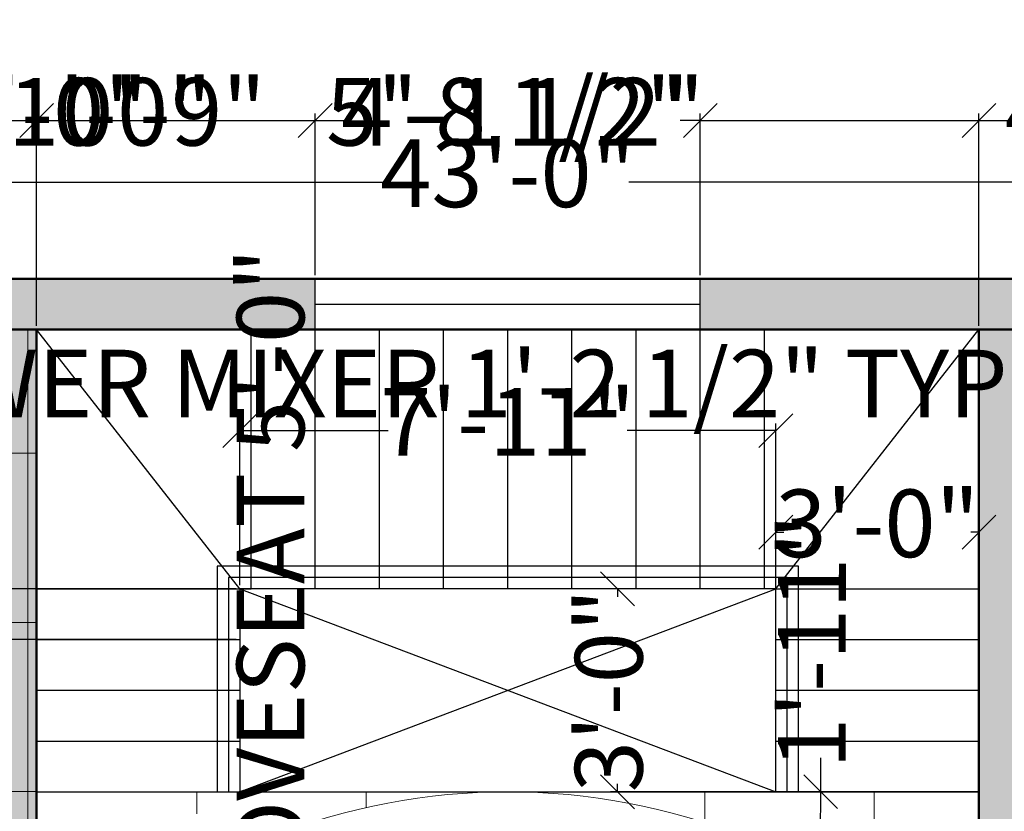
# Model space of a CAD drawing. Units: inches. Extents: x 2371 to 3019, y 129 to 700.
# Tile 9 of 14: x 2579 to 2753, y 537 to 677. Entities that reach past the tile are written whole.
import ezdxf

# ---------------------------------------------------------------- set-up
doc = ezdxf.new("R2010")
doc.units = ezdxf.units.IN
for name, color, linetype, lineweight in [('A-ANNO-DIMS', 2, 'Continuous', 18), ('A-FLOR-PATT', 252, 'Continuous', 13), ('A-FLOR-STRS', 3, 'Continuous', 25), ('A-FURN', 8, 'Continuous', 18), ('A-GLAZ', 4, 'Continuous', 25), ('A-WALL', 7, 'Continuous', 50), ('A-WALL-PATT', 8, 'Continuous', 13)]:
    doc.layers.add(name, color=color, linetype=linetype, lineweight=lineweight)
doc.styles.get("Standard").update_dxf_attribs({"font": 'arial.ttf'})
doc.dimstyles.new('ISO-25', dxfattribs={"dimtxt": 12, "dimasz": 6, "dimexe": 1.25, "dimexo": 0.625, "dimtad": 0, "dimdec": 1, "dimlunit": 3, "dimtxsty": 'Standard', "dimblk": 'OBLIQUE', "dimblk1": 'ORIGIN2', "dimblk2": 'OBLIQUE', "dimcen": 2.5, "dimadec": 0, "dimazin": 0, "dimtfac": 1, "dimtdec": 1, "dimtmove": 0, "dimatfit": 3, "dimldrblk": 'OBLIQUE', "dimfxl": 1, "dimarcsym": 0})

# ---------------------------------------------------------------- blocks, each defined once
blk = doc.blocks.new('Sofa - Roundback 7 ft.')
for p, q in [((-12.00002, -32.4421), (-12.00003, -6.5971)), ((11.99997, -32.4421), (11.99998, -6.5971)), ((-36.000027, -34), (-36.000027, -11.4696)), ((35.99998, -34), (35.99998, -11.4696)), ((-35.999844, -13.3819), (35.9998, -13.3819)), ((-36.000027, -32.4421), (35.99998, -32.4421))]:
    blk.add_line(p, q)
for points in [[(-36.000027, -34), (-42.000027, -34), (-42.000027, -8)], [(41.99998, -8), (41.99998, -34), (35.99998, -34)]]:
    blk.add_lwpolyline(points)
for centre, radius, start, end in [((0, -114.25), 114.25, 68.43141, 111.5686), ((-0.00001, -127.1968), 121.1968, 72.72033, 107.2797)]:
    blk.add_arc(centre, radius, start, end)
blk = doc.blocks.new('_Oblique')
at = {"color": 0, "linetype": 'ByBlock', "lineweight": -2}
blk.add_line((-0.5, -0.5), (0.5, 0.5), dxfattribs=at)
blk = doc.blocks.new('*D14')
at = {"layer": 'A-ANNO-DIMS', "color": 0, "lineweight": -2, "transparency": 16777216}
for p, q in [((2407.11, 631.6), (2407.11, 649.37)), ((2923.11, 631.6), (2923.11, 649.37)), ((2407.11, 648.12), (2643.63, 648.12)), ((2923.11, 648.12), (2686.58, 648.12))]:
    blk.add_line(p, q, dxfattribs=at)
at = {"layer": 'Defpoints', "color": 0, "lineweight": 25, "transparency": 16777216}
for p in [(2923.11, 648.12), (2407.11, 630.98), (2923.11, 630.98)]:
    blk.add_point(p, dxfattribs=at)
at = {"layer": 'A-ANNO-DIMS', "color": 0, "lineweight": -2, "transparency": 16777216, "xscale": 6, "yscale": 6, "zscale": 6, "rotation": 180}
blk.add_blockref('_Oblique', (2407.11, 648.12), dxfattribs=at)
at = {"layer": 'A-ANNO-DIMS', "color": 0, "lineweight": -2, "transparency": 16777216, "xscale": 6, "yscale": 6, "zscale": 6}
blk.add_blockref('_Oblique', (2923.11, 648.12), dxfattribs=at)
at = {"layer": 'A-ANNO-DIMS', "color": 0, "transparency": 16777216, "insert": (2665.11, 648.12), "char_height": 12, "width": 20.8486, "attachment_point": 5}
blk.add_mtext('43\'-0"', dxfattribs=at)
blk = doc.blocks.new('_Origin2')
at = {"color": 0, "linetype": 'ByBlock', "lineweight": -2}
blk.add_line((-0.5, 0), (-1, 0), dxfattribs=at)
for radius in [0.5, 0.25]:
    blk.add_circle((0, 0), radius, dxfattribs=at)
blk = doc.blocks.new('*D30')
at = {"layer": 'A-ANNO-DIMS', "color": 0, "lineweight": -2, "transparency": 16777216}
for p, q in [((2505.18, 612.41), (2505.18, 609.58)), ((2505.18, 610.83), (2519.88, 610.83)), ((2519.88, 612.41), (2519.88, 609.58)), ((2519.88, 610.83), (2525.88, 610.83))]:
    blk.add_line(p, q, dxfattribs=at)
at = {"layer": 'Defpoints', "color": 0, "lineweight": 25, "transparency": 16777216}
for p in [(2505.18, 613.03), (2519.88, 613.03), (2519.88, 610.83)]:
    blk.add_point(p, dxfattribs=at)
at = {"layer": 'A-ANNO-DIMS', "color": 0, "lineweight": -2, "transparency": 16777216, "xscale": 6, "yscale": 6, "zscale": 6, "rotation": 180}
blk.add_blockref('_Oblique', (2505.18, 610.83), dxfattribs=at)
at = {"layer": 'A-ANNO-DIMS', "color": 0, "lineweight": -2, "transparency": 16777216, "xscale": 6, "yscale": 6, "zscale": 6}
blk.add_blockref('_Oblique', (2519.88, 610.83), dxfattribs=at)
at = {"layer": 'A-ANNO-DIMS', "color": 0, "transparency": 16777216, "insert": (2645.95, 610.83), "char_height": 12, "attachment_point": 5}
blk.add_mtext('SHOWER MIXER 1\'-2 1/2" TYP.', dxfattribs=at)
blk = doc.blocks.new('*D32')
at = {"layer": 'A-ANNO-DIMS', "color": 0, "lineweight": -2, "transparency": 16777216}
for p, q in [((2624.61, 507.98), (2624.61, 513.98)), ((2616.23, 507.98), (2625.86, 507.98)), ((2624.61, 447.98), (2624.61, 507.98)), ((2616.23, 447.98), (2625.86, 447.98))]:
    blk.add_line(p, q, dxfattribs=at)
at = {"layer": 'Defpoints', "color": 0, "lineweight": 25, "transparency": 16777216}
for p in [(2615.61, 507.98), (2624.61, 507.98), (2615.61, 447.98)]:
    blk.add_point(p, dxfattribs=at)
at = {"layer": 'A-ANNO-DIMS', "color": 0, "lineweight": -2, "transparency": 16777216, "xscale": 6, "yscale": 6, "zscale": 6}
for p, rotation in [((2624.61, 507.98), 90), ((2624.61, 447.98), 270)]:
    blk.add_blockref('_Oblique', p, dxfattribs=dict(at, rotation=rotation))
at = {"layer": 'A-ANNO-DIMS', "color": 0, "transparency": 16777216, "insert": (2624.61, 576.87), "char_height": 12, "attachment_point": 5, "rotation": 90}
blk.add_mtext('LOVESEAT 5\'-0"', dxfattribs=at)
blk = doc.blocks.new('*D38')
at = {"layer": 'A-ANNO-DIMS', "color": 0, "lineweight": -2, "transparency": 16777216}
for p, q in [((2536.61, 631.6), (2536.61, 660.28)), ((2560.61, 631.6), (2560.61, 660.28)), ((2536.61, 659.03), (2560.61, 659.03)), ((2560.61, 659.03), (2566.61, 659.03))]:
    blk.add_line(p, q, dxfattribs=at)
at = {"layer": 'Defpoints', "color": 0, "lineweight": 25, "transparency": 16777216}
for p in [(2560.61, 659.03), (2536.61, 630.98), (2560.61, 630.98)]:
    blk.add_point(p, dxfattribs=at)
at = {"layer": 'A-ANNO-DIMS', "color": 0, "lineweight": -2, "transparency": 16777216, "xscale": 6, "yscale": 6, "zscale": 6, "rotation": 180}
blk.add_blockref('_Oblique', (2536.61, 659.03), dxfattribs=at)
at = {"layer": 'A-ANNO-DIMS', "color": 0, "lineweight": -2, "transparency": 16777216, "xscale": 6, "yscale": 6, "zscale": 6}
blk.add_blockref('_Oblique', (2560.61, 659.03), dxfattribs=at)
at = {"layer": 'A-ANNO-DIMS', "color": 0, "transparency": 16777216, "insert": (2583.28, 659.03), "char_height": 12, "attachment_point": 5}
blk.add_mtext('2\'-0"', dxfattribs=at)
blk = doc.blocks.new('*D39')
at = {"layer": 'A-ANNO-DIMS', "color": 0, "lineweight": -2, "transparency": 16777216}
for p, q in [((2560.61, 631.6), (2560.61, 660.28)), ((2572.61, 622.6), (2572.61, 660.28)), ((2560.61, 659.03), (2572.61, 659.03)), ((2572.61, 659.03), (2578.61, 659.03))]:
    blk.add_line(p, q, dxfattribs=at)
at = {"layer": 'Defpoints', "color": 0, "lineweight": 25, "transparency": 16777216}
for p in [(2572.61, 659.03), (2560.61, 630.98), (2572.61, 621.98)]:
    blk.add_point(p, dxfattribs=at)
at = {"layer": 'A-ANNO-DIMS', "color": 0, "lineweight": -2, "transparency": 16777216, "xscale": 6, "yscale": 6, "zscale": 6, "rotation": 180}
blk.add_blockref('_Oblique', (2560.61, 659.03), dxfattribs=at)
at = {"layer": 'A-ANNO-DIMS', "color": 0, "lineweight": -2, "transparency": 16777216, "xscale": 6, "yscale": 6, "zscale": 6}
blk.add_blockref('_Oblique', (2572.61, 659.03), dxfattribs=at)
at = {"layer": 'A-ANNO-DIMS', "color": 0, "transparency": 16777216, "insert": (2594.61, 659.03), "char_height": 12, "attachment_point": 5}
blk.add_mtext('1\'-0"', dxfattribs=at)
blk = doc.blocks.new('*D40')
at = {"layer": 'A-ANNO-DIMS', "color": 0, "lineweight": -2, "transparency": 16777216}
for p, q in [((2572.61, 622.6), (2572.61, 660.28)), ((2581.61, 622.6), (2581.61, 660.28)), ((2572.61, 659.03), (2581.61, 659.03)), ((2581.61, 659.03), (2587.61, 659.03))]:
    blk.add_line(p, q, dxfattribs=at)
at = {"layer": 'Defpoints', "color": 0, "lineweight": 25, "transparency": 16777216}
for p in [(2581.61, 659.03), (2572.61, 621.98), (2581.61, 621.98)]:
    blk.add_point(p, dxfattribs=at)
at = {"layer": 'A-ANNO-DIMS', "color": 0, "lineweight": -2, "transparency": 16777216, "xscale": 6, "yscale": 6, "zscale": 6, "rotation": 180}
blk.add_blockref('_Oblique', (2572.61, 659.03), dxfattribs=at)
at = {"layer": 'A-ANNO-DIMS', "color": 0, "lineweight": -2, "transparency": 16777216, "xscale": 6, "yscale": 6, "zscale": 6}
blk.add_blockref('_Oblique', (2581.61, 659.03), dxfattribs=at)
at = {"layer": 'A-ANNO-DIMS', "color": 0, "transparency": 16777216, "insert": (2604.18, 659.03), "char_height": 12, "attachment_point": 5}
blk.add_mtext('0\'-9"', dxfattribs=at)
blk = doc.blocks.new('*D41')
at = {"layer": 'A-ANNO-DIMS', "color": 0, "lineweight": -2, "transparency": 16777216}
for p, q in [((2581.61, 622.6), (2581.61, 660.28)), ((2630.98, 631.6), (2630.98, 660.28)), ((2581.61, 659.03), (2630.98, 659.03)), ((2630.98, 659.03), (2636.98, 659.03))]:
    blk.add_line(p, q, dxfattribs=at)
at = {"layer": 'Defpoints', "color": 0, "lineweight": 25, "transparency": 16777216}
for p in [(2630.98, 659.03), (2630.98, 630.98), (2581.61, 621.98)]:
    blk.add_point(p, dxfattribs=at)
at = {"layer": 'A-ANNO-DIMS', "color": 0, "lineweight": -2, "transparency": 16777216, "xscale": 6, "yscale": 6, "zscale": 6, "rotation": 180}
blk.add_blockref('_Oblique', (2581.61, 659.03), dxfattribs=at)
at = {"layer": 'A-ANNO-DIMS', "color": 0, "lineweight": -2, "transparency": 16777216, "xscale": 6, "yscale": 6, "zscale": 6}
blk.add_blockref('_Oblique', (2630.98, 659.03), dxfattribs=at)
at = {"layer": 'A-ANNO-DIMS', "color": 0, "transparency": 16777216, "insert": (2667.78, 659.03), "char_height": 12, "attachment_point": 5}
blk.add_mtext('4\'-1 1/2"', dxfattribs=at)
blk = doc.blocks.new('*D42')
at = {"layer": 'A-ANNO-DIMS', "color": 0, "lineweight": -2, "transparency": 16777216}
for p, q in [((2630.98, 631.6), (2630.98, 660.28)), ((2699.23, 631.6), (2699.23, 660.28)), ((2630.98, 659.03), (2634.55, 659.03)), ((2699.23, 659.03), (2695.66, 659.03))]:
    blk.add_line(p, q, dxfattribs=at)
at = {"layer": 'Defpoints', "color": 0, "lineweight": 25, "transparency": 16777216}
for p in [(2699.23, 659.03), (2630.98, 630.98), (2699.23, 630.98)]:
    blk.add_point(p, dxfattribs=at)
at = {"layer": 'A-ANNO-DIMS', "color": 0, "lineweight": -2, "transparency": 16777216, "xscale": 6, "yscale": 6, "zscale": 6, "rotation": 180}
blk.add_blockref('_Oblique', (2630.98, 659.03), dxfattribs=at)
at = {"layer": 'A-ANNO-DIMS', "color": 0, "lineweight": -2, "transparency": 16777216, "xscale": 6, "yscale": 6, "zscale": 6}
blk.add_blockref('_Oblique', (2699.23, 659.03), dxfattribs=at)
at = {"layer": 'A-ANNO-DIMS', "color": 0, "transparency": 16777216, "insert": (2665.11, 659.03), "char_height": 12, "attachment_point": 5}
blk.add_mtext('5\'-8 1/2"', dxfattribs=at)
blk = doc.blocks.new('*D43')
at = {"layer": 'A-ANNO-DIMS', "color": 0, "lineweight": -2, "transparency": 16777216}
for p, q in [((2699.23, 631.6), (2699.23, 660.28)), ((2748.61, 622.6), (2748.61, 660.28)), ((2699.23, 659.03), (2748.61, 659.03)), ((2748.61, 659.03), (2754.61, 659.03))]:
    blk.add_line(p, q, dxfattribs=at)
at = {"layer": 'Defpoints', "color": 0, "lineweight": 25, "transparency": 16777216}
for p in [(2748.61, 659.03), (2699.23, 630.98), (2748.61, 621.98)]:
    blk.add_point(p, dxfattribs=at)
at = {"layer": 'A-ANNO-DIMS', "color": 0, "lineweight": -2, "transparency": 16777216, "xscale": 6, "yscale": 6, "zscale": 6, "rotation": 180}
blk.add_blockref('_Oblique', (2699.23, 659.03), dxfattribs=at)
at = {"layer": 'A-ANNO-DIMS', "color": 0, "lineweight": -2, "transparency": 16777216, "xscale": 6, "yscale": 6, "zscale": 6}
blk.add_blockref('_Oblique', (2748.61, 659.03), dxfattribs=at)
at = {"layer": 'A-ANNO-DIMS', "color": 0, "transparency": 16777216, "insert": (2785.4, 659.03), "char_height": 12, "attachment_point": 5}
blk.add_mtext('4\'-1 1/2"', dxfattribs=at)
blk = doc.blocks.new('*D44')
at = {"layer": 'A-ANNO-DIMS', "color": 0, "lineweight": -2, "transparency": 16777216}
for p, q in [((2748.61, 622.6), (2748.61, 660.28)), ((2757.61, 622.6), (2757.61, 660.28)), ((2748.61, 659.03), (2757.61, 659.03)), ((2757.61, 659.03), (2763.61, 659.03))]:
    blk.add_line(p, q, dxfattribs=at)
at = {"layer": 'Defpoints', "color": 0, "lineweight": 25, "transparency": 16777216}
for p in [(2757.61, 659.03), (2748.61, 621.98), (2757.61, 621.98)]:
    blk.add_point(p, dxfattribs=at)
at = {"layer": 'A-ANNO-DIMS', "color": 0, "lineweight": -2, "transparency": 16777216, "xscale": 6, "yscale": 6, "zscale": 6, "rotation": 180}
blk.add_blockref('_Oblique', (2748.61, 659.03), dxfattribs=at)
at = {"layer": 'A-ANNO-DIMS', "color": 0, "lineweight": -2, "transparency": 16777216, "xscale": 6, "yscale": 6, "zscale": 6}
blk.add_blockref('_Oblique', (2757.61, 659.03), dxfattribs=at)
at = {"layer": 'A-ANNO-DIMS', "color": 0, "transparency": 16777216, "insert": (2780.18, 659.03), "char_height": 12, "attachment_point": 5}
blk.add_mtext('0\'-9"', dxfattribs=at)
blk = doc.blocks.new('*D65')
at = {"layer": 'A-ANNO-DIMS', "color": 0, "lineweight": -2, "transparency": 16777216}
for p, q in [((2618.98, 621.98), (2377.81, 621.98)), ((2379.06, 621.98), (2379.06, 620.21)), ((2379.06, 575.98), (2379.06, 577.74)), ((2616.98, 575.98), (2377.81, 575.98))]:
    blk.add_line(p, q, dxfattribs=at)
at = {"layer": 'Defpoints', "color": 0, "lineweight": 25, "transparency": 16777216}
for p in [(2379.06, 621.98), (2619.61, 621.98), (2617.61, 575.98)]:
    blk.add_point(p, dxfattribs=at)
at = {"layer": 'A-ANNO-DIMS', "color": 0, "lineweight": -2, "transparency": 16777216, "xscale": 6, "yscale": 6, "zscale": 6}
for p, rotation in [((2379.06, 621.98), 90), ((2379.06, 575.98), 270)]:
    blk.add_blockref('_Oblique', p, dxfattribs=dict(at, rotation=rotation))
at = {"layer": 'A-ANNO-DIMS', "color": 0, "transparency": 16777216, "insert": (2379.06, 598.98), "char_height": 12, "attachment_point": 5, "rotation": 90}
blk.add_mtext('3\'-10"', dxfattribs=at)
blk = doc.blocks.new('*D66')
at = {"layer": 'A-ANNO-DIMS', "color": 0, "lineweight": -2, "transparency": 16777216}
for p, q in [((2711.98, 575.98), (2683.31, 575.98)), ((2684.56, 575.98), (2684.56, 574.55)), ((2684.56, 539.98), (2684.56, 541.41)), ((2711.98, 539.98), (2683.31, 539.98))]:
    blk.add_line(p, q, dxfattribs=at)
at = {"layer": 'Defpoints', "color": 0, "lineweight": 25, "transparency": 16777216}
for p in [(2684.56, 575.98), (2712.61, 575.98), (2712.61, 539.98)]:
    blk.add_point(p, dxfattribs=at)
at = {"layer": 'A-ANNO-DIMS', "color": 0, "lineweight": -2, "transparency": 16777216, "xscale": 6, "yscale": 6, "zscale": 6}
for p, rotation in [((2684.56, 575.98), 90), ((2684.56, 539.98), 270)]:
    blk.add_blockref('_Oblique', p, dxfattribs=dict(at, rotation=rotation))
at = {"layer": 'A-ANNO-DIMS', "color": 0, "transparency": 16777216, "insert": (2684.56, 557.98), "char_height": 12, "attachment_point": 5, "rotation": 90}
blk.add_mtext('3\'-0"', dxfattribs=at)
blk = doc.blocks.new('*D67')
at = {"layer": 'A-ANNO-DIMS', "color": 0, "lineweight": -2, "transparency": 16777216}
for p, q in [((2379.06, 575.98), (2379.06, 581.98)), ((2616.98, 575.98), (2377.81, 575.98)), ((2379.06, 566.98), (2379.06, 575.98)), ((2616.98, 566.98), (2377.81, 566.98))]:
    blk.add_line(p, q, dxfattribs=at)
at = {"layer": 'Defpoints', "color": 0, "lineweight": 25, "transparency": 16777216}
for p in [(2379.06, 575.98), (2617.61, 575.98), (2617.61, 566.98)]:
    blk.add_point(p, dxfattribs=at)
at = {"layer": 'A-ANNO-DIMS', "color": 0, "lineweight": -2, "transparency": 16777216, "xscale": 6, "yscale": 6, "zscale": 6}
for p, rotation in [((2379.06, 575.98), 90), ((2379.06, 566.98), 270)]:
    blk.add_blockref('_Oblique', p, dxfattribs=dict(at, rotation=rotation))
at = {"layer": 'A-ANNO-DIMS', "color": 0, "transparency": 16777216, "insert": (2379.06, 598.55), "char_height": 12, "attachment_point": 5, "rotation": 90}
blk.add_mtext('0\'-9"', dxfattribs=at)
blk = doc.blocks.new('*D68')
at = {"layer": 'A-ANNO-DIMS', "color": 0, "lineweight": -2, "transparency": 16777216}
for p, q in [((2617.61, 576.6), (2617.61, 605.28)), ((2617.61, 604.03), (2643.92, 604.03)), ((2712.61, 604.03), (2686.29, 604.03)), ((2712.61, 576.6), (2712.61, 605.28))]:
    blk.add_line(p, q, dxfattribs=at)
at = {"layer": 'Defpoints', "color": 0, "lineweight": 25, "transparency": 16777216}
for p in [(2712.61, 604.03), (2617.61, 575.98), (2712.61, 575.98)]:
    blk.add_point(p, dxfattribs=at)
at = {"layer": 'A-ANNO-DIMS', "color": 0, "lineweight": -2, "transparency": 16777216, "xscale": 6, "yscale": 6, "zscale": 6, "rotation": 180}
blk.add_blockref('_Oblique', (2617.61, 604.03), dxfattribs=at)
at = {"layer": 'A-ANNO-DIMS', "color": 0, "lineweight": -2, "transparency": 16777216, "xscale": 6, "yscale": 6, "zscale": 6}
blk.add_blockref('_Oblique', (2712.61, 604.03), dxfattribs=at)
at = {"layer": 'A-ANNO-DIMS', "color": 0, "transparency": 16777216, "insert": (2665.11, 604.03), "char_height": 12, "attachment_point": 5}
blk.add_mtext('7\'-11"', dxfattribs=at)
blk = doc.blocks.new('*D69')
at = {"layer": 'A-ANNO-DIMS', "color": 0, "lineweight": -2, "transparency": 16777216}
for p, q in [((2712.61, 558.6), (2712.61, 587.28)), ((2748.61, 558.6), (2748.61, 587.28)), ((2712.61, 586.03), (2714.03, 586.03)), ((2748.61, 586.03), (2747.18, 586.03))]:
    blk.add_line(p, q, dxfattribs=at)
at = {"layer": 'Defpoints', "color": 0, "lineweight": 25, "transparency": 16777216}
for p in [(2748.61, 586.03), (2712.61, 557.98), (2748.61, 557.98)]:
    blk.add_point(p, dxfattribs=at)
at = {"layer": 'A-ANNO-DIMS', "color": 0, "lineweight": -2, "transparency": 16777216, "xscale": 6, "yscale": 6, "zscale": 6, "rotation": 180}
blk.add_blockref('_Oblique', (2712.61, 586.03), dxfattribs=at)
at = {"layer": 'A-ANNO-DIMS', "color": 0, "lineweight": -2, "transparency": 16777216, "xscale": 6, "yscale": 6, "zscale": 6}
blk.add_blockref('_Oblique', (2748.61, 586.03), dxfattribs=at)
at = {"layer": 'A-ANNO-DIMS', "color": 0, "transparency": 16777216, "insert": (2730.61, 586.03), "char_height": 12, "attachment_point": 5}
blk.add_mtext('3\'-0"', dxfattribs=at)
blk = doc.blocks.new('*D73')
at = {"layer": 'A-ANNO-DIMS', "color": 0, "lineweight": -2, "transparency": 16777216}
for p, q in [((2720.56, 540), (2720.56, 546)), ((2747.98, 539.98), (2719.31, 540)), ((2720.54, 517.01), (2720.56, 540)), ((2747.96, 516.99), (2719.29, 517.01))]:
    blk.add_line(p, q, dxfattribs=at)
at = {"layer": 'Defpoints', "color": 0, "lineweight": 25, "transparency": 16777216}
for p in [(2720.56, 540), (2748.61, 539.98), (2748.59, 516.99)]:
    blk.add_point(p, dxfattribs=at)
at = {"layer": 'A-ANNO-DIMS', "color": 0, "lineweight": -2, "transparency": 16777216, "xscale": 6, "yscale": 6, "zscale": 6}
for p, rotation in [((2720.56, 540), 89.96084939784976), ((2720.54, 517.01), 269.9608493978498)]:
    blk.add_blockref('_Oblique', p, dxfattribs=dict(at, rotation=rotation))
at = {"layer": 'A-ANNO-DIMS', "color": 0, "transparency": 16777216, "insert": (2720.57, 566.67), "char_height": 12, "attachment_point": 5, "rotation": 89.9608}
blk.add_mtext('1\'-11"', dxfattribs=at)

msp = doc.modelspace()

# ---------------------------------------------------------------- hatches: boundary and pattern name
at = {"layer": 'A-FLOR-PATT'}
h = msp.add_hatch(dxfattribs=at)
h.set_pattern_fill('_USER', color=256, scale=30, pattern_type=0)
h.set_pattern_definition([(0, (0, 0), (0, 30), [])])
h.paths.add_polyline_path([(2913.11, 498.98), (2827.61, 498.98), (2827.61, 531.98), (2832.11, 531.98), (2832.11, 537.98), (2833.61, 537.98), (2833.61, 605.98), (2818.35, 605.98, -1), (2796.86, 605.98), (2781.61, 605.98), (2781.61, 603.98), (2781.61, 533.98), (2757.61, 533.98), (2757.61, 531.98), (2797.61, 531.98), (2797.61, 522.98), (2757.61, 522.98), (2757.61, 516.98), (2754.59, 516.98), (2772.52, 485.76), (2771.01, 484.89), (2770.98, 484.93, -0.097552), (2757.61, 481.1), (2757.61, 422.48), (2837.61, 422.48), (2837.61, 362.48), (2757.61, 362.48), (2757.61, 303.98), (2835.86, 303.98, -0.09439), (2793.86, 311.98), (2793.86, 337.98), (2799.86, 337.98), (2799.86, 336.42), (2871.86, 336.42), (2871.86, 337.98), (2877.86, 337.98), (2877.86, 311.98, -0.09439), (2835.86, 303.98), (2913.11, 303.98), (2913.11, 383.18), (2904.11, 383.18), (2904.11, 419.18), (2913.11, 419.18)])
h.paths.add_polyline_path([(2788.88, 332.88), (2788.88, 308.88), (2764.88, 308.88), (2764.88, 332.88)], flags=16)
h.paths.add_polyline_path([(2788.4, 325.04, -1), (2774.4, 325.04, -1)], flags=0)
h.paths.add_polyline_path([(2781.4, 328.04), (2784.4, 325.04), (2781.4, 322.04), (2778.4, 325.04)], flags=0)
h.paths.add_polyline_path([(2782.4, 325.04, -1), (2780.4, 325.04, -1)], flags=0)
h.paths.add_polyline_path([(2748.61, 480.99), (2754.51, 480.98, 0.119303), (2770.98, 484.93), (2753.07, 516.1), (2754.59, 516.98), (2748.61, 516.98), (2748.61, 539.98), (2712.61, 539.98), (2665.11, 539.98, -0.09439), (2707.11, 531.98), (2707.11, 505.98), (2701.11, 505.98), (2701.11, 507.53), (2629.11, 507.53), (2629.11, 505.98), (2623.11, 505.98), (2623.11, 531.98, -0.09439), (2665.11, 539.98), (2581.61, 539.98), (2581.61, 522.98), (2581.61, 477.98, -0.131044), (2589.61, 507.98), (2615.61, 507.98), (2615.61, 501.98), (2614.05, 501.98), (2614.05, 453.98), (2615.61, 453.98), (2615.61, 447.98), (2589.61, 447.98, -0.131044), (2581.61, 477.98), (2581.61, 432.98), (2572.61, 432.98, 0.119303), (2556.14, 428.99), (2574.12, 397.85), (2572.61, 396.98), (2578.61, 396.98), (2581.61, 396.98), (2581.61, 390.98), (2748.61, 390.98)])
h.paths.add_polyline_path([(2683.1, 447.25), (2652.43, 447.25), (2652.43, 492.22), (2683.1, 492.22)], flags=16)
h.paths.add_polyline_path([(2682.1, 448.25), (2653.43, 448.25), (2653.43, 491.22), (2682.1, 491.22)], flags=0)
h.paths.add_polyline_path([(2613.58, 512.06), (2589.58, 512.06), (2589.58, 536.06), (2613.58, 536.06)], flags=16)
h.paths.add_polyline_path([(2599.1, 528.22, -1), (2613.1, 528.22, -1)], flags=0)
h.paths.add_polyline_path([(2609.1, 528.22), (2606.1, 525.22), (2603.1, 528.22), (2606.1, 531.22)], flags=0)
h.paths.add_polyline_path([(2607.1, 528.22, -1), (2605.1, 528.22, -1)], flags=0)
h.paths.add_polyline_path([(2581.61, 522.98), (2581.61, 621.98), (2572.61, 621.98), (2572.61, 522.98), (2572.61, 500.98), (2565.85, 500.98), (2565.85, 500.15), (2564.82, 500.15), (2561.16, 500.19), (2561.16, 500.17), (2560.13, 500.3), (2560.22, 500.98), (2556.38, 500.98), (2556.43, 500.22), (2555.4, 500.14), (2555.34, 500.98), (2551.07, 500.98), (2551.07, 500.15), (2550.04, 500.15), (2547.64, 500.19), (2547.64, 500.15), (2546.61, 500.15), (2541.79, 500.22), (2540.72, 500.13), (2540.65, 500.98), (2533.37, 500.98), (2533.37, 500.15), (2532.34, 500.15), (2529.13, 500.21), (2529.12, 500.13), (2528.09, 500.22), (2528.16, 500.98), (2523.23, 500.98), (2523.23, 500.15), (2522.2, 500.15), (2519.8, 500.21), (2519.8, 500.15), (2518.77, 500.15), (2514.45, 500.26), (2514.44, 500.14), (2513.41, 500.22), (2513.47, 500.98), (2509.62, 500.98), (2509.71, 500.3), (2508.69, 500.17), (2508.58, 500.98), (2505.03, 500.98), (2505.03, 500.15), (2503.99, 500.15), (2501.07, 500.29), (2501.07, 500.15), (2500.04, 500.15), (2496.44, 500.37), (2496.44, 500.15), (2495.4, 500.15), (2492.55, 500.41), (2492.18, 500.35), (2492.09, 500.98), (2486.11, 500.98), (2486.11, 524.98), (2486.11, 531.98), (2490.61, 531.98), (2490.61, 537.98), (2492.11, 537.98), (2492.11, 605.98), (2476.85, 605.98, -1), (2455.36, 605.98), (2440.11, 605.98), (2440.11, 533.98), (2416.11, 533.98), (2416.11, 605.98), (2416.11, 621.98), (2536.61, 621.98), (2536.61, 630.98), (2407.11, 630.98), (2407.11, 363.98), (2416.11, 363.98), (2416.11, 431.48), (2496.11, 431.48), (2496.11, 371.48), (2416.11, 371.48), (2416.11, 303.98), (2494.36, 303.98, -0.09439), (2452.36, 311.98), (2452.36, 337.98), (2458.36, 337.98), (2458.36, 336.42), (2530.36, 336.42), (2530.36, 337.98), (2536.36, 337.98), (2536.36, 311.98, -0.09439), (2494.36, 303.98), (2572.61, 303.98), (2572.61, 381.98), (2572.61, 396.98), (2554.61, 428.15), (2556.12, 429.03), (2556.14, 428.99, -0.119303), (2572.61, 432.98), (2578.61, 432.98), (2581.61, 432.98)])
h.paths.add_polyline_path([(2450.11, 500.98), (2444.5, 500.98), (2444.44, 500.14), (2443.41, 500.22), (2443.47, 500.98), (2439.62, 500.98), (2439.71, 500.3), (2438.69, 500.17), (2438.58, 500.98), (2435.02, 500.98), (2435.02, 500.15), (2433.99, 500.15), (2433.99, 500.98), (2431.07, 500.98), (2431.07, 500.15), (2430.04, 500.15), (2430.04, 500.98), (2426.43, 500.98), (2426.43, 500.15), (2425.4, 500.15), (2425.4, 500.98), (2423.13, 500.98), (2423.2, 500.5), (2422.18, 500.35), (2422.09, 500.98), (2416.11, 500.98), (2416.11, 524.98), (2416.11, 531.98), (2450.11, 531.98), (2450.11, 522.98)], flags=16)
h.paths.add_polyline_path([(2449.11, 501.98), (2417.11, 501.98), (2417.11, 522.98), (2417.11, 523.98), (2449.11, 523.98)], flags=0)
h.paths.add_polyline_path([(2420.7, 510.73), (2419.36, 520.07), (2420.38, 520.22), (2421.74, 510.73), (2425.4, 510.73), (2425.4, 520.07), (2426.43, 520.07), (2426.43, 510.73), (2430.04, 510.73), (2430.04, 520.07), (2431.07, 520.07), (2431.07, 510.73), (2433.99, 510.73), (2433.99, 520.07), (2435.02, 520.07), (2435.02, 510.73), (2437.35, 510.73), (2436.18, 519.93), (2437.2, 520.06), (2438.39, 510.73), (2444.17, 510.73), (2444.85, 520.08), (2445.88, 520.01), (2445.21, 510.73)], flags=0)
h.paths.add_polyline_path([(2446.94, 336.11), (2446.94, 312.11), (2422.94, 312.11), (2422.94, 336.11)], flags=16)
h.paths.add_polyline_path([(2446.46, 328.27, -1), (2432.46, 328.27, -1)], flags=0)
h.paths.add_polyline_path([(2439.46, 331.27), (2442.46, 328.27), (2439.46, 325.27), (2436.46, 328.27)], flags=0)
h.paths.add_polyline_path([(2440.46, 328.27, -1), (2438.46, 328.27, -1)], flags=0)
h.paths.add_polyline_path([(2816, 444.88), (2866.87, 444.88), (2866.87, 463.54), (2816, 463.54)], flags=24)
h.paths.add_polyline_path([(2794.21, 558.3), (2833.34, 558.3), (2833.34, 576.96), (2794.21, 576.96)], flags=24)
h.paths.add_polyline_path([(2651.69, 411.53), (2711.04, 411.53), (2711.04, 430.19), (2651.69, 430.19)], flags=24)
h.paths.add_polyline_path([(2494.09, 444.88), (2544.97, 444.88), (2544.97, 463.54), (2494.09, 463.54)], flags=24)
h.paths.add_polyline_path([(2444.55, 565.02), (2483.69, 565.02), (2483.69, 583.68), (2444.55, 583.68)], flags=24)
h = msp.add_hatch(dxfattribs=at)
h.set_pattern_fill('_USER', color=256, scale=30, angle=90, pattern_type=0)
h.set_pattern_definition([(90, (0, 0), (-30, 2e-15), [])])
h.paths.add_polyline_path([(2913.11, 498.98), (2827.61, 498.98), (2827.61, 531.98), (2832.11, 531.98), (2832.11, 537.98), (2833.61, 537.98), (2833.61, 605.98), (2818.35, 605.98, -1), (2796.86, 605.98), (2781.61, 605.98), (2781.61, 603.98), (2781.61, 533.98), (2757.61, 533.98), (2757.61, 531.98), (2797.61, 531.98), (2797.61, 522.98), (2757.61, 522.98), (2757.61, 516.98), (2754.59, 516.98), (2772.52, 485.76), (2771.01, 484.89), (2770.98, 484.93, -0.097552), (2757.61, 481.1), (2757.61, 422.48), (2837.61, 422.48), (2837.61, 362.48), (2757.61, 362.48), (2757.61, 303.98), (2835.86, 303.98, -0.09439), (2793.86, 311.98), (2793.86, 337.98), (2799.86, 337.98), (2799.86, 336.42), (2871.86, 336.42), (2871.86, 337.98), (2877.86, 337.98), (2877.86, 311.98, -0.09439), (2835.86, 303.98), (2913.11, 303.98), (2913.11, 383.18), (2904.11, 383.18), (2904.11, 419.18), (2913.11, 419.18)])
h.paths.add_polyline_path([(2788.88, 332.88), (2788.88, 308.88), (2764.88, 308.88), (2764.88, 332.88)], flags=16)
h.paths.add_polyline_path([(2788.4, 325.04, -1), (2774.4, 325.04, -1)], flags=0)
h.paths.add_polyline_path([(2781.4, 328.04), (2784.4, 325.04), (2781.4, 322.04), (2778.4, 325.04)], flags=0)
h.paths.add_polyline_path([(2782.4, 325.04, -1), (2780.4, 325.04, -1)], flags=0)
h.paths.add_polyline_path([(2748.61, 480.99), (2754.51, 480.98, 0.119303), (2770.98, 484.93), (2753.07, 516.1), (2754.59, 516.98), (2748.61, 516.98), (2748.61, 539.98), (2712.61, 539.98), (2665.11, 539.98, -0.09439), (2707.11, 531.98), (2707.11, 505.98), (2701.11, 505.98), (2701.11, 507.53), (2629.11, 507.53), (2629.11, 505.98), (2623.11, 505.98), (2623.11, 531.98, -0.09439), (2665.11, 539.98), (2581.61, 539.98), (2581.61, 522.98), (2581.61, 477.98, -0.131044), (2589.61, 507.98), (2615.61, 507.98), (2615.61, 501.98), (2614.05, 501.98), (2614.05, 453.98), (2615.61, 453.98), (2615.61, 447.98), (2589.61, 447.98, -0.131044), (2581.61, 477.98), (2581.61, 432.98), (2572.61, 432.98, 0.119303), (2556.14, 428.99), (2574.12, 397.85), (2572.61, 396.98), (2578.61, 396.98), (2581.61, 396.98), (2581.61, 390.98), (2748.61, 390.98)])
h.paths.add_polyline_path([(2683.1, 447.25), (2652.43, 447.25), (2652.43, 492.22), (2683.1, 492.22)], flags=16)
h.paths.add_polyline_path([(2682.1, 448.25), (2653.43, 448.25), (2653.43, 491.22), (2682.1, 491.22)], flags=0)
h.paths.add_polyline_path([(2613.58, 512.06), (2589.58, 512.06), (2589.58, 536.06), (2613.58, 536.06)], flags=16)
h.paths.add_polyline_path([(2599.1, 528.22, -1), (2613.1, 528.22, -1)], flags=0)
h.paths.add_polyline_path([(2609.1, 528.22), (2606.1, 525.22), (2603.1, 528.22), (2606.1, 531.22)], flags=0)
h.paths.add_polyline_path([(2607.1, 528.22, -1), (2605.1, 528.22, -1)], flags=0)
h.paths.add_polyline_path([(2581.61, 522.98), (2581.61, 621.98), (2572.61, 621.98), (2572.61, 522.98), (2572.61, 500.98), (2565.85, 500.98), (2565.85, 500.15), (2564.82, 500.15), (2561.16, 500.19), (2561.16, 500.17), (2560.13, 500.3), (2560.22, 500.98), (2556.38, 500.98), (2556.43, 500.22), (2555.4, 500.14), (2555.34, 500.98), (2551.07, 500.98), (2551.07, 500.15), (2550.04, 500.15), (2547.64, 500.19), (2547.64, 500.15), (2546.61, 500.15), (2541.79, 500.22), (2540.72, 500.13), (2540.65, 500.98), (2533.37, 500.98), (2533.37, 500.15), (2532.34, 500.15), (2529.13, 500.21), (2529.12, 500.13), (2528.09, 500.22), (2528.16, 500.98), (2523.23, 500.98), (2523.23, 500.15), (2522.2, 500.15), (2519.8, 500.21), (2519.8, 500.15), (2518.77, 500.15), (2514.45, 500.26), (2514.44, 500.14), (2513.41, 500.22), (2513.47, 500.98), (2509.62, 500.98), (2509.71, 500.3), (2508.69, 500.17), (2508.58, 500.98), (2505.03, 500.98), (2505.03, 500.15), (2503.99, 500.15), (2501.07, 500.29), (2501.07, 500.15), (2500.04, 500.15), (2496.44, 500.37), (2496.44, 500.15), (2495.4, 500.15), (2492.55, 500.41), (2492.18, 500.35), (2492.09, 500.98), (2486.11, 500.98), (2486.11, 524.98), (2486.11, 531.98), (2490.61, 531.98), (2490.61, 537.98), (2492.11, 537.98), (2492.11, 605.98), (2476.85, 605.98, -1), (2455.36, 605.98), (2440.11, 605.98), (2440.11, 533.98), (2416.11, 533.98), (2416.11, 605.98), (2416.11, 621.98), (2536.61, 621.98), (2536.61, 630.98), (2407.11, 630.98), (2407.11, 363.98), (2416.11, 363.98), (2416.11, 431.48), (2496.11, 431.48), (2496.11, 371.48), (2416.11, 371.48), (2416.11, 303.98), (2494.36, 303.98, -0.09439), (2452.36, 311.98), (2452.36, 337.98), (2458.36, 337.98), (2458.36, 336.42), (2530.36, 336.42), (2530.36, 337.98), (2536.36, 337.98), (2536.36, 311.98, -0.09439), (2494.36, 303.98), (2572.61, 303.98), (2572.61, 381.98), (2572.61, 396.98), (2554.61, 428.15), (2556.12, 429.03), (2556.14, 428.99, -0.119303), (2572.61, 432.98), (2578.61, 432.98), (2581.61, 432.98)])
h.paths.add_polyline_path([(2450.11, 500.98), (2444.5, 500.98), (2444.44, 500.14), (2443.41, 500.22), (2443.47, 500.98), (2439.62, 500.98), (2439.71, 500.3), (2438.69, 500.17), (2438.58, 500.98), (2435.02, 500.98), (2435.02, 500.15), (2433.99, 500.15), (2433.99, 500.98), (2431.07, 500.98), (2431.07, 500.15), (2430.04, 500.15), (2430.04, 500.98), (2426.43, 500.98), (2426.43, 500.15), (2425.4, 500.15), (2425.4, 500.98), (2423.13, 500.98), (2423.2, 500.5), (2422.18, 500.35), (2422.09, 500.98), (2416.11, 500.98), (2416.11, 524.98), (2416.11, 531.98), (2450.11, 531.98), (2450.11, 522.98)], flags=16)
h.paths.add_polyline_path([(2449.11, 501.98), (2417.11, 501.98), (2417.11, 522.98), (2417.11, 523.98), (2449.11, 523.98)], flags=0)
h.paths.add_polyline_path([(2420.7, 510.73), (2419.36, 520.07), (2420.38, 520.22), (2421.74, 510.73), (2425.4, 510.73), (2425.4, 520.07), (2426.43, 520.07), (2426.43, 510.73), (2430.04, 510.73), (2430.04, 520.07), (2431.07, 520.07), (2431.07, 510.73), (2433.99, 510.73), (2433.99, 520.07), (2435.02, 520.07), (2435.02, 510.73), (2437.35, 510.73), (2436.18, 519.93), (2437.2, 520.06), (2438.39, 510.73), (2444.17, 510.73), (2444.85, 520.08), (2445.88, 520.01), (2445.21, 510.73)], flags=0)
h.paths.add_polyline_path([(2446.94, 336.11), (2446.94, 312.11), (2422.94, 312.11), (2422.94, 336.11)], flags=16)
h.paths.add_polyline_path([(2446.46, 328.27, -1), (2432.46, 328.27, -1)], flags=0)
h.paths.add_polyline_path([(2439.46, 331.27), (2442.46, 328.27), (2439.46, 325.27), (2436.46, 328.27)], flags=0)
h.paths.add_polyline_path([(2440.46, 328.27, -1), (2438.46, 328.27, -1)], flags=0)
h.paths.add_polyline_path([(2816, 444.88), (2866.87, 444.88), (2866.87, 463.54), (2816, 463.54)], flags=24)
h.paths.add_polyline_path([(2794.21, 558.3), (2833.34, 558.3), (2833.34, 576.96), (2794.21, 576.96)], flags=24)
h.paths.add_polyline_path([(2651.69, 411.53), (2711.04, 411.53), (2711.04, 430.19), (2651.69, 430.19)], flags=24)
h.paths.add_polyline_path([(2494.09, 444.88), (2544.97, 444.88), (2544.97, 463.54), (2494.09, 463.54)], flags=24)
h.paths.add_polyline_path([(2444.55, 565.02), (2483.69, 565.02), (2483.69, 583.68), (2444.55, 583.68)], flags=24)
at = {"layer": 'A-WALL-PATT'}
h = msp.add_hatch(color=256, dxfattribs=at)
h.dxf.hatch_style = 1
h.paths.add_polyline_path([(2536.61, 630.98), (2407.11, 630.98), (2407.11, 363.98), (2416.11, 363.98), (2416.11, 498.98), (2416.11, 522.98), (2416.11, 531.98), (2416.11, 603.98), (2416.11, 621.98), (2536.61, 621.98)])
h.paths.add_polyline_path([(2630.98, 630.98), (2560.61, 630.98), (2560.61, 621.98), (2630.98, 621.98)])
h.paths.add_polyline_path([(2878.11, 630.98), (2699.23, 630.98), (2699.23, 621.98), (2878.11, 621.98)])
h.paths.add_polyline_path([(2496.61, 621.98), (2492.11, 621.98), (2492.11, 569.98), (2496.61, 569.98)], flags=17)
h.paths.add_polyline_path([(2581.61, 621.98), (2572.61, 621.98), (2572.61, 522.98), (2572.61, 498.98), (2572.61, 432.98), (2578.61, 432.98), (2581.61, 432.98), (2581.61, 522.98)])
h.paths.add_polyline_path([(2572.61, 531.98), (2486.11, 531.98), (2486.11, 522.98), (2572.61, 522.98)])
h.paths.add_polyline_path([(2450.11, 531.98), (2440.11, 531.98), (2416.11, 531.98), (2416.11, 522.98), (2450.11, 522.98)], flags=17)
h.paths.add_polyline_path([(2416.11, 315.98), (2407.11, 315.98), (2407.11, 294.98), (2458.11, 294.98), (2458.11, 303.98), (2416.11, 303.98)])
h.paths.add_polyline_path([(2757.61, 303.98), (2530.61, 303.98), (2530.61, 294.98), (2757.61, 294.98)])
h.paths.add_polyline_path([(2581.61, 381.98), (2605.61, 381.98), (2617.61, 381.98), (2617.61, 390.98), (2581.61, 390.98), (2581.61, 396.98), (2572.61, 396.98), (2572.61, 381.98), (2572.61, 303.98), (2581.61, 303.98)])
h.paths.add_polyline_path([(2757.61, 480.98), (2748.61, 480.98), (2748.61, 381.98), (2748.61, 303.98), (2757.61, 303.98), (2757.61, 381.98), (2757.61, 422.48)])
h.paths.add_polyline_path([(2797.61, 531.98), (2757.61, 531.98), (2757.61, 603.98), (2757.61, 621.98), (2748.61, 621.98), (2748.61, 516.99), (2754.59, 516.98), (2757.61, 516.98), (2757.61, 522.98), (2797.61, 522.98)])
h.paths.add_polyline_path([(2913.11, 531.98), (2827.61, 531.98), (2827.61, 522.98), (2913.11, 522.98)])
h.paths.add_polyline_path([(2923.11, 630.98), (2902.11, 630.98), (2902.11, 621.98), (2914.11, 621.98), (2914.11, 363.98), (2923.11, 363.98)])
h.paths.add_polyline_path([(2923.11, 315.98), (2914.11, 315.98), (2914.11, 303.98), (2866.11, 303.98), (2866.11, 294.98), (2923.11, 294.98)])
h.paths.add_polyline_path([(2793.61, 303.98), (2757.61, 303.98), (2757.61, 294.98), (2793.61, 294.98)])

# ---------------------------------------------------------------- linework, layer by layer
at = {"layer": 'A-FLOR-STRS'}
for p, q in [((2630.98, 575.98), (2630.98, 630.98)), ((2699.23, 575.98), (2699.23, 630.98)), ((2617.61, 575.98), (2581.61, 621.98)), ((2619.61, 575.98), (2619.61, 621.98)), ((2642.36, 575.98), (2642.36, 621.98)), ((2653.73, 575.98), (2653.73, 621.98)), ((2665.11, 575.98), (2665.11, 621.98)), ((2676.48, 575.98), (2676.48, 621.98)), ((2687.86, 575.98), (2687.86, 621.98)), ((2710.61, 575.98), (2710.61, 621.98)), ((2712.61, 575.98), (2748.61, 621.98)), ((2581.61, 575.98), (2617.61, 575.98)), ((2617.61, 575.98), (2619.61, 575.98)), ((2712.61, 575.98), (2710.61, 575.98)), ((2712.61, 575.98), (2748.61, 575.98)), ((2581.61, 566.98), (2617.61, 566.98)), ((2712.61, 566.98), (2748.61, 566.98)), ((2581.61, 557.98), (2617.61, 557.98)), ((2712.61, 557.98), (2748.61, 557.98)), ((2581.61, 548.98), (2617.61, 548.98)), ((2712.61, 548.98), (2748.61, 548.98)), ((2581.61, 539.98), (2748.61, 539.98)), ((2581.61, 539.98), (2617.61, 539.98)), ((2748.61, 539.98), (2712.61, 539.98))]:
    msp.add_line(p, q, dxfattribs=at)
at = {"layer": 'A-FLOR-STRS', "ltscale": 0.2}
for p, q in [((2617.61, 575.98), (2712.61, 539.98)), ((2617.61, 539.98), (2712.61, 575.98))]:
    msp.add_line(p, q, dxfattribs=at)
at = {"layer": 'A-FLOR-STRS'}
for points in [[(2716.61, 539.98), (2716.61, 579.98), (2613.61, 579.98), (2613.61, 539.98)], [(2714.61, 539.98), (2714.61, 577.98), (2615.61, 577.98), (2615.61, 539.98)], [(2712.61, 539.98), (2712.61, 575.98), (2617.61, 575.98), (2617.61, 539.98)]]:
    msp.add_lwpolyline(points, dxfattribs=at)
at = {"layer": 'A-GLAZ'}
msp.add_line((2630.98, 626.48), (2699.23, 626.48), dxfattribs=at)
at = {"layer": 'A-WALL'}
for p, q in [((2878.11, 630.98), (2560.61, 630.98)), ((2878.11, 621.98), (2560.61, 621.98)), ((2581.61, 621.98), (2581.61, 522.98)), ((2748.61, 516.99), (2748.61, 621.98))]:
    msp.add_line(p, q, dxfattribs=at)

# ---------------------------------------------------------------- block references
at = {"layer": 'A-FURN'}
msp.add_blockref('Sofa - Roundback 7 ft.', (2665.11, 539.98), dxfattribs=at)

# ---------------------------------------------------------------- dimensions: what is measured, and where the dimension line sits
at = {"layer": 'A-ANNO-DIMS'}
for base, p1, p2, picture, middle in [((2630.98, 659.03), (2581.61, 621.98), (2630.98, 630.98), '*D41', (2667.78, 659.03)), ((2699.2301, 659.026162), (2630.9801, 630.976162), (2699.2301, 630.976162), '*D42', (2665.1051, 659.026162)), ((2748.61, 659.03), (2699.23, 630.98), (2748.61, 621.98), '*D43', (2785.4, 659.03)), ((2560.61, 659.03), (2536.61, 630.98), (2560.61, 630.98), '*D38', (2583.28, 659.03)), ((2572.61, 659.03), (2560.61, 630.98), (2572.61, 621.98), '*D39', (2594.61, 659.03)), ((2581.61, 659.03), (2572.61, 621.98), (2581.61, 621.98), '*D40', (2604.18, 659.03)), ((2757.61, 659.03), (2748.61, 621.98), (2757.61, 621.98), '*D44', (2780.18, 659.03)), ((2712.61, 604.03), (2617.61, 575.98), (2712.61, 575.98), '*D68', (2665.11, 604.03)), ((2748.61, 586.03), (2712.61, 557.98), (2748.61, 557.98), '*D69', (2730.61, 586.03))]:
    dim = msp.add_linear_dim(base=base, p1=p1, p2=p2, dimstyle='ISO-25', override={"dimdec": 1, "dimlfac": 1, "dimrnd": 0, "dimzin": 1, "dimdsep": 46, "dimlunit": 4, "dimfrac": 2}, dxfattribs=at)
    dim.commit()
    dim.dimension.update_dxf_attribs({"geometry": picture, "text_midpoint": middle})
for base, p1, p2, text, override, picture, middle in [((2519.88, 610.83), (2505.18, 613.03), (2519.88, 613.03), 'SHOWER MIXER <> TYP.', {"dimdec": 1, "dimrnd": 0, "dimzin": 1, "dimlunit": 4, "dimfrac": 2}, '*D30', (2645.95, 610.83)), ((2923.11, 648.12), (2407.11, 630.98), (2923.11, 630.98), '43\'-0"', {"dimclrd": 0, "dimclre": 0, "dimclrt": 0}, '*D14', (2665.11, 648.12))]:
    dim = msp.add_linear_dim(base=base, p1=p1, p2=p2, text=text, dimstyle='ISO-25', override=override, dxfattribs=at)
    dim.commit()
    dim.dimension.update_dxf_attribs({"geometry": picture, "text_midpoint": middle})
dim = msp.add_linear_dim(base=(2624.61, 507.98), p1=(2615.61, 447.98), p2=(2615.61, 507.98), angle=90, text='LOVESEAT <>', dimstyle='ISO-25', override={"dimdec": 1, "dimrnd": 0, "dimzin": 1, "dimlunit": 4, "dimfrac": 2}, dxfattribs=at)
dim.commit()
dim.dimension.update_dxf_attribs({"geometry": '*D32', "text_midpoint": (2624.61, 576.87)})
for base, p1, p2, angle, picture, middle in [((2379.06, 621.98), (2617.61, 575.98), (2619.61, 621.98), 90, '*D65', (2379.06, 598.98)), ((2379.06, 575.98), (2617.61, 566.98), (2617.61, 575.98), 90, '*D67', (2379.06, 598.55)), ((2720.56, 540), (2748.59, 516.99), (2748.61, 539.98), 89.9608, '*D73', (2720.57, 566.67)), ((2684.56, 575.98), (2712.61, 539.98), (2712.61, 575.98), 90, '*D66', (2684.56, 557.98))]:
    dim = msp.add_linear_dim(base=base, p1=p1, p2=p2, angle=angle, dimstyle='ISO-25', override={"dimdec": 1, "dimlfac": 1, "dimrnd": 0, "dimzin": 1, "dimdsep": 46, "dimlunit": 4, "dimfrac": 2}, dxfattribs=at)
    dim.commit()
    dim.dimension.update_dxf_attribs({"geometry": picture, "text_midpoint": middle})

doc.saveas('drawing.dxf')
